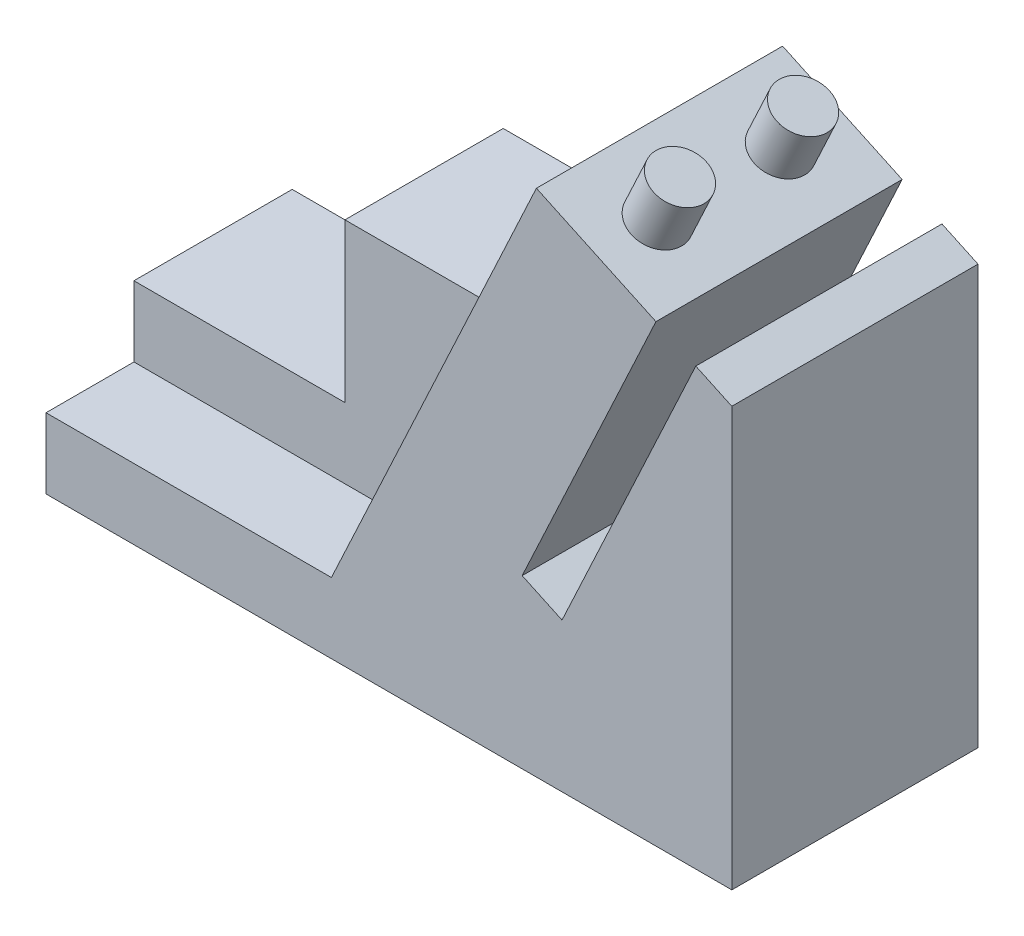
ISO-10303-21;
HEADER;
FILE_DESCRIPTION(('STEP AP214'),'2;1');
FILE_NAME('part.step','',(''),(''),'','','');
FILE_SCHEMA(('AUTOMOTIVE_DESIGN { 1 0 10303 214 1 1 1 1 }'));
ENDSEC;
DATA;
#1=APPLICATION_CONTEXT('core data for automotive mechanical design processes');
#2=APPLICATION_PROTOCOL_DEFINITION('international standard','automotive_design',2000,#1);
#3=PRODUCT_CONTEXT('',#1,'mechanical');
#4=PRODUCT('Part','Part','',(#3));
#5=PRODUCT_RELATED_PRODUCT_CATEGORY('part','',(#4));
#6=PRODUCT_DEFINITION_FORMATION('','',#4);
#7=PRODUCT_DEFINITION_CONTEXT('part definition',#1,'design');
#8=PRODUCT_DEFINITION('design','',#6,#7);
#9=PRODUCT_DEFINITION_SHAPE('','',#8);
#10=(LENGTH_UNIT() NAMED_UNIT(*) SI_UNIT(.MILLI.,.METRE.));
#11=(NAMED_UNIT(*) PLANE_ANGLE_UNIT() SI_UNIT($,.RADIAN.));
#12=(NAMED_UNIT(*) SI_UNIT($,.STERADIAN.) SOLID_ANGLE_UNIT());
#13=UNCERTAINTY_MEASURE_WITH_UNIT(LENGTH_MEASURE(1.E-05),#10,'distance_accuracy_value','');
#14=(GEOMETRIC_REPRESENTATION_CONTEXT(3) GLOBAL_UNCERTAINTY_ASSIGNED_CONTEXT((#13)) GLOBAL_UNIT_ASSIGNED_CONTEXT((#10,
#11,#12)) REPRESENTATION_CONTEXT('',''));
#15=CARTESIAN_POINT('',(0.,0.,0.));
#16=DIRECTION('',(0.,0.,1.));
#17=DIRECTION('',(1.,0.,0.));
#18=AXIS2_PLACEMENT_3D('',#15,#16,#17);
#19=CARTESIAN_POINT('',(78.,0.,28.));
#20=DIRECTION('',(0.,1.,0.));
#21=DIRECTION('',(0.,0.,1.));
#22=AXIS2_PLACEMENT_3D('',#19,#20,#21);
#23=PLANE('',#22);
#24=DIRECTION('',(1.,0.,0.));
#25=VECTOR('',#24,1.);
#26=CARTESIAN_POINT('',(78.,0.,0.));
#27=LINE('',#26,#25);
#28=CARTESIAN_POINT('',(0.,0.,0.));
#29=VERTEX_POINT('',#28);
#30=CARTESIAN_POINT('',(78.,0.,0.));
#31=VERTEX_POINT('',#30);
#32=EDGE_CURVE('E182',#29,#31,#27,.T.);
#33=ORIENTED_EDGE('',*,*,#32,.T.);
#34=DIRECTION('',(0.,0.,-1.));
#35=VECTOR('',#34,1.);
#36=CARTESIAN_POINT('',(78.,0.,28.));
#37=LINE('',#36,#35);
#38=CARTESIAN_POINT('',(78.,0.,28.));
#39=VERTEX_POINT('',#38);
#40=EDGE_CURVE('E249',#39,#31,#37,.T.);
#41=ORIENTED_EDGE('',*,*,#40,.F.);
#42=DIRECTION('',(1.,0.,0.));
#43=VECTOR('',#42,1.);
#44=CARTESIAN_POINT('',(78.,0.,28.));
#45=LINE('',#44,#43);
#46=CARTESIAN_POINT('',(0.,0.,28.));
#47=VERTEX_POINT('',#46);
#48=EDGE_CURVE('E183',#47,#39,#45,.T.);
#49=ORIENTED_EDGE('',*,*,#48,.F.);
#50=DIRECTION('',(0.,0.,-1.));
#51=VECTOR('',#50,1.);
#52=CARTESIAN_POINT('',(0.,0.,28.));
#53=LINE('',#52,#51);
#54=EDGE_CURVE('E207',#47,#29,#53,.T.);
#55=ORIENTED_EDGE('',*,*,#54,.T.);
#56=EDGE_LOOP('',(#33,#41,#49,#55));
#57=FACE_BOUND('',#56,.T.);
#58=ADVANCED_FACE('F39',(#57),#23,.F.);
#59=CARTESIAN_POINT('',(78.,47.6371964383334,28.));
#60=DIRECTION('',(-1.,0.,0.));
#61=DIRECTION('',(0.,0.,1.));
#62=AXIS2_PLACEMENT_3D('',#59,#60,#61);
#63=PLANE('',#62);
#64=DIRECTION('',(0.,1.,0.));
#65=VECTOR('',#64,1.);
#66=CARTESIAN_POINT('',(78.,47.6371964383334,0.));
#67=LINE('',#66,#65);
#68=CARTESIAN_POINT('',(78.,47.6371964383334,0.));
#69=VERTEX_POINT('',#68);
#70=EDGE_CURVE('E209',#31,#69,#67,.T.);
#71=ORIENTED_EDGE('',*,*,#70,.T.);
#72=DIRECTION('',(0.,0.,-1.));
#73=VECTOR('',#72,1.);
#74=CARTESIAN_POINT('',(78.,47.6371964383334,28.));
#75=LINE('',#74,#73);
#76=CARTESIAN_POINT('',(78.,47.6371964383334,28.));
#77=VERTEX_POINT('',#76);
#78=EDGE_CURVE('E250',#77,#69,#75,.T.);
#79=ORIENTED_EDGE('',*,*,#78,.F.);
#80=DIRECTION('',(0.,1.,0.));
#81=VECTOR('',#80,1.);
#82=CARTESIAN_POINT('',(78.,47.6371964383334,28.));
#83=LINE('',#82,#81);
#84=EDGE_CURVE('E190',#39,#77,#83,.T.);
#85=ORIENTED_EDGE('',*,*,#84,.F.);
#86=ORIENTED_EDGE('',*,*,#40,.T.);
#87=EDGE_LOOP('',(#71,#79,#85,#86));
#88=FACE_BOUND('',#87,.T.);
#89=ADVANCED_FACE('F309',(#88),#63,.F.);
#90=CARTESIAN_POINT('',(73.9030517868581,49.5476347651859,28.));
#91=DIRECTION('',(-0.422618261740702,-0.906307787036649,0.));
#92=DIRECTION('',(0.906307787036649,-0.422618261740702,0.));
#93=AXIS2_PLACEMENT_3D('',#90,#91,#92);
#94=PLANE('',#93);
#95=DIRECTION('',(-0.906307787036649,0.422618261740702,0.));
#96=VECTOR('',#95,1.);
#97=CARTESIAN_POINT('',(73.9030517868581,49.5476347651859,0.));
#98=LINE('',#97,#96);
#99=CARTESIAN_POINT('',(73.9030517868581,49.5476347651859,0.));
#100=VERTEX_POINT('',#99);
#101=EDGE_CURVE('E212',#69,#100,#98,.T.);
#102=ORIENTED_EDGE('',*,*,#101,.T.);
#103=DIRECTION('',(0.,0.,-1.));
#104=VECTOR('',#103,1.);
#105=CARTESIAN_POINT('',(73.9030517868581,49.5476347651859,28.));
#106=LINE('',#105,#104);
#107=CARTESIAN_POINT('',(73.9030517868581,49.5476347651859,28.));
#108=VERTEX_POINT('',#107);
#109=EDGE_CURVE('E242',#108,#100,#106,.T.);
#110=ORIENTED_EDGE('',*,*,#109,.F.);
#111=DIRECTION('',(-0.906307787036649,0.422618261740702,0.));
#112=VECTOR('',#111,1.);
#113=CARTESIAN_POINT('',(73.9030517868581,49.5476347651859,28.));
#114=LINE('',#113,#112);
#115=EDGE_CURVE('E188',#77,#108,#114,.T.);
#116=ORIENTED_EDGE('',*,*,#115,.F.);
#117=ORIENTED_EDGE('',*,*,#78,.T.);
#118=EDGE_LOOP('',(#102,#110,#116,#117));
#119=FACE_BOUND('',#118,.T.);
#120=ADVANCED_FACE('F304',(#119),#94,.F.);
#121=CARTESIAN_POINT('',(58.6887943641928,16.9205544318666,28.));
#122=DIRECTION('',(0.906307787036648,-0.422618261740703,0.));
#123=DIRECTION('',(0.422618261740703,0.906307787036648,0.));
#124=AXIS2_PLACEMENT_3D('',#121,#122,#123);
#125=PLANE('',#124);
#126=DIRECTION('',(-0.422618261740703,-0.906307787036648,0.));
#127=VECTOR('',#126,1.);
#128=CARTESIAN_POINT('',(58.6887943641928,16.9205544318666,0.));
#129=LINE('',#128,#127);
#130=CARTESIAN_POINT('',(58.6887943641928,16.9205544318666,0.));
#131=VERTEX_POINT('',#130);
#132=EDGE_CURVE('E214',#100,#131,#129,.T.);
#133=ORIENTED_EDGE('',*,*,#132,.T.);
#134=DIRECTION('',(0.,0.,-1.));
#135=VECTOR('',#134,1.);
#136=CARTESIAN_POINT('',(58.6887943641928,16.9205544318666,28.));
#137=LINE('',#136,#135);
#138=CARTESIAN_POINT('',(58.6887943641928,16.9205544318666,28.));
#139=VERTEX_POINT('',#138);
#140=EDGE_CURVE('E241',#139,#131,#137,.T.);
#141=ORIENTED_EDGE('',*,*,#140,.F.);
#142=DIRECTION('',(-0.422618261740703,-0.906307787036648,0.));
#143=VECTOR('',#142,1.);
#144=CARTESIAN_POINT('',(58.6887943641928,16.9205544318666,28.));
#145=LINE('',#144,#143);
#146=EDGE_CURVE('E195',#108,#139,#145,.T.);
#147=ORIENTED_EDGE('',*,*,#146,.F.);
#148=ORIENTED_EDGE('',*,*,#109,.T.);
#149=EDGE_LOOP('',(#133,#141,#147,#148));
#150=FACE_BOUND('',#149,.T.);
#151=ADVANCED_FACE('F301',(#150),#125,.F.);
#152=CARTESIAN_POINT('',(54.1572554290096,19.0336457405701,28.));
#153=DIRECTION('',(-0.422618261740703,-0.906307787036648,0.));
#154=DIRECTION('',(0.906307787036648,-0.422618261740703,0.));
#155=AXIS2_PLACEMENT_3D('',#152,#153,#154);
#156=PLANE('',#155);
#157=DIRECTION('',(-0.906307787036648,0.422618261740703,0.));
#158=VECTOR('',#157,1.);
#159=CARTESIAN_POINT('',(54.1572554290096,19.0336457405701,0.));
#160=LINE('',#159,#158);
#161=CARTESIAN_POINT('',(54.1572554290096,19.0336457405701,0.));
#162=VERTEX_POINT('',#161);
#163=EDGE_CURVE('E213',#131,#162,#160,.T.);
#164=ORIENTED_EDGE('',*,*,#163,.T.);
#165=DIRECTION('',(0.,0.,-1.));
#166=VECTOR('',#165,1.);
#167=CARTESIAN_POINT('',(54.1572554290096,19.0336457405701,28.));
#168=LINE('',#167,#166);
#169=CARTESIAN_POINT('',(54.1572554290096,19.0336457405701,28.));
#170=VERTEX_POINT('',#169);
#171=EDGE_CURVE('E238',#170,#162,#168,.T.);
#172=ORIENTED_EDGE('',*,*,#171,.F.);
#173=DIRECTION('',(-0.906307787036648,0.422618261740703,0.));
#174=VECTOR('',#173,1.);
#175=CARTESIAN_POINT('',(54.1572554290096,19.0336457405701,28.));
#176=LINE('',#175,#174);
#177=EDGE_CURVE('E191',#139,#170,#176,.T.);
#178=ORIENTED_EDGE('',*,*,#177,.F.);
#179=ORIENTED_EDGE('',*,*,#140,.T.);
#180=EDGE_LOOP('',(#164,#172,#178,#179));
#181=FACE_BOUND('',#180,.T.);
#182=ADVANCED_FACE('F300',(#181),#156,.F.);
#183=CARTESIAN_POINT('',(69.3715128516749,51.6607260738894,28.));
#184=DIRECTION('',(-0.906307787036648,0.422618261740704,0.));
#185=DIRECTION('',(-0.422618261740704,-0.906307787036648,0.));
#186=AXIS2_PLACEMENT_3D('',#183,#184,#185);
#187=PLANE('',#186);
#188=DIRECTION('',(0.422618261740704,0.906307787036648,0.));
#189=VECTOR('',#188,1.);
#190=CARTESIAN_POINT('',(69.3715128516749,51.6607260738894,0.));
#191=LINE('',#190,#189);
#192=CARTESIAN_POINT('',(69.3715128516749,51.6607260738894,0.));
#193=VERTEX_POINT('',#192);
#194=EDGE_CURVE('E219',#162,#193,#191,.T.);
#195=ORIENTED_EDGE('',*,*,#194,.T.);
#196=DIRECTION('',(0.,0.,-1.));
#197=VECTOR('',#196,1.);
#198=CARTESIAN_POINT('',(69.3715128516749,51.6607260738894,28.));
#199=LINE('',#198,#197);
#200=CARTESIAN_POINT('',(69.3715128516749,51.6607260738894,28.));
#201=VERTEX_POINT('',#200);
#202=EDGE_CURVE('E232',#201,#193,#199,.T.);
#203=ORIENTED_EDGE('',*,*,#202,.F.);
#204=DIRECTION('',(0.422618261740704,0.906307787036648,0.));
#205=VECTOR('',#204,1.);
#206=CARTESIAN_POINT('',(69.3715128516749,51.6607260738894,28.));
#207=LINE('',#206,#205);
#208=EDGE_CURVE('E198',#170,#201,#207,.T.);
#209=ORIENTED_EDGE('',*,*,#208,.F.);
#210=ORIENTED_EDGE('',*,*,#171,.T.);
#211=EDGE_LOOP('',(#195,#203,#209,#210));
#212=FACE_BOUND('',#211,.T.);
#213=ADVANCED_FACE('F263',(#212),#187,.F.);
#214=CARTESIAN_POINT('',(55.7768960461252,58.,28.));
#215=DIRECTION('',(-0.422618261740704,-0.906307787036648,0.));
#216=DIRECTION('',(0.906307787036648,-0.422618261740704,0.));
#217=AXIS2_PLACEMENT_3D('',#214,#215,#216);
#218=PLANE('',#217);
#219=CARTESIAN_POINT('',(62.5742044489,54.8303630369447,7.));
#220=DIRECTION('',(-0.422618261740704,-0.906307787036648,0.));
#221=DIRECTION('',(0.906307787036648,-0.422618261740704,0.));
#222=AXIS2_PLACEMENT_3D('',#219,#220,#221);
#223=CIRCLE('',#222,3.00000000000001);
#224=CARTESIAN_POINT('',(65.29312781001,53.5625082517226,7.));
#225=VERTEX_POINT('',#224);
#226=EDGE_CURVE('E11',#225,#225,#223,.F.);
#227=ORIENTED_EDGE('',*,*,#226,.F.);
#228=EDGE_LOOP('',(#227));
#229=FACE_BOUND('',#228,.T.);
#230=CARTESIAN_POINT('',(62.5742044489,54.8303630369447,21.));
#231=DIRECTION('',(-0.422618261740704,-0.906307787036648,0.));
#232=DIRECTION('',(0.906307787036648,-0.422618261740704,0.));
#233=AXIS2_PLACEMENT_3D('',#230,#231,#232);
#234=CIRCLE('',#233,3.);
#235=CARTESIAN_POINT('',(65.29312781001,53.5625082517226,21.));
#236=VERTEX_POINT('',#235);
#237=EDGE_CURVE('E46',#236,#236,#234,.F.);
#238=ORIENTED_EDGE('',*,*,#237,.F.);
#239=EDGE_LOOP('',(#238));
#240=FACE_BOUND('',#239,.T.);
#241=DIRECTION('',(-0.906307787036648,0.422618261740704,0.));
#242=VECTOR('',#241,1.);
#243=CARTESIAN_POINT('',(55.7768960461252,58.,0.));
#244=LINE('',#243,#242);
#245=CARTESIAN_POINT('',(55.7768960461252,58.,0.));
#246=VERTEX_POINT('',#245);
#247=EDGE_CURVE('E220',#193,#246,#244,.T.);
#248=ORIENTED_EDGE('',*,*,#247,.T.);
#249=DIRECTION('',(0.,0.,-1.));
#250=VECTOR('',#249,1.);
#251=CARTESIAN_POINT('',(55.7768960461252,58.,28.));
#252=LINE('',#251,#250);
#253=CARTESIAN_POINT('',(55.7768960461252,58.,28.));
#254=VERTEX_POINT('',#253);
#255=EDGE_CURVE('E235',#254,#246,#252,.T.);
#256=ORIENTED_EDGE('',*,*,#255,.F.);
#257=DIRECTION('',(-0.906307787036648,0.422618261740704,0.));
#258=VECTOR('',#257,1.);
#259=CARTESIAN_POINT('',(55.7768960461252,58.,28.));
#260=LINE('',#259,#258);
#261=EDGE_CURVE('E197',#201,#254,#260,.T.);
#262=ORIENTED_EDGE('',*,*,#261,.F.);
#263=ORIENTED_EDGE('',*,*,#202,.T.);
#264=EDGE_LOOP('',(#248,#256,#262,#263));
#265=FACE_BOUND('',#264,.T.);
#266=ADVANCED_FACE('F260',(#229,#240,#265),#218,.F.);
#267=CARTESIAN_POINT('',(32.461513138375,8.,28.));
#268=DIRECTION('',(0.906307787036648,-0.422618261740704,0.));
#269=DIRECTION('',(0.422618261740704,0.906307787036648,0.));
#270=AXIS2_PLACEMENT_3D('',#267,#268,#269);
#271=PLANE('',#270);
#272=DIRECTION('',(0.,0.,1.));
#273=VECTOR('',#272,1.);
#274=CARTESIAN_POINT('',(44.5855122504051,34.,28.));
#275=LINE('',#274,#273);
#276=CARTESIAN_POINT('',(44.5855122504051,34.,0.));
#277=VERTEX_POINT('',#276);
#278=CARTESIAN_POINT('',(44.5855122504051,34.,18.));
#279=VERTEX_POINT('',#278);
#280=EDGE_CURVE('E163',#277,#279,#275,.T.);
#281=ORIENTED_EDGE('',*,*,#280,.T.);
#282=DIRECTION('',(0.422618261740704,0.906307787036648,0.));
#283=VECTOR('',#282,1.);
#284=CARTESIAN_POINT('',(37.5311484498391,18.8718680098944,18.));
#285=LINE('',#284,#283);
#286=CARTESIAN_POINT('',(32.461513138375,8.,18.));
#287=VERTEX_POINT('',#286);
#288=EDGE_CURVE('E62',#287,#279,#285,.T.);
#289=ORIENTED_EDGE('',*,*,#288,.F.);
#290=DIRECTION('',(0.,0.,-1.));
#291=VECTOR('',#290,1.);
#292=CARTESIAN_POINT('',(32.461513138375,8.,28.));
#293=LINE('',#292,#291);
#294=CARTESIAN_POINT('',(32.461513138375,8.,28.));
#295=VERTEX_POINT('',#294);
#296=EDGE_CURVE('E229',#295,#287,#293,.T.);
#297=ORIENTED_EDGE('',*,*,#296,.F.);
#298=DIRECTION('',(-0.422618261740704,-0.906307787036648,0.));
#299=VECTOR('',#298,1.);
#300=CARTESIAN_POINT('',(32.461513138375,8.,28.));
#301=LINE('',#300,#299);
#302=EDGE_CURVE('E196',#254,#295,#301,.T.);
#303=ORIENTED_EDGE('',*,*,#302,.F.);
#304=ORIENTED_EDGE('',*,*,#255,.T.);
#305=DIRECTION('',(-0.422618261740704,-0.906307787036648,0.));
#306=VECTOR('',#305,1.);
#307=CARTESIAN_POINT('',(32.461513138375,8.,0.));
#308=LINE('',#307,#306);
#309=EDGE_CURVE('E221',#246,#277,#308,.T.);
#310=ORIENTED_EDGE('',*,*,#309,.T.);
#311=EDGE_LOOP('',(#281,#289,#297,#303,#304,#310));
#312=FACE_BOUND('',#311,.T.);
#313=ADVANCED_FACE('F258',(#312),#271,.F.);
#314=CARTESIAN_POINT('',(0.,8.,28.));
#315=DIRECTION('',(0.,-1.,0.));
#316=DIRECTION('',(0.,0.,-1.));
#317=AXIS2_PLACEMENT_3D('',#314,#315,#316);
#318=PLANE('',#317);
#319=ORIENTED_EDGE('',*,*,#296,.T.);
#320=DIRECTION('',(1.,0.,0.));
#321=VECTOR('',#320,1.);
#322=CARTESIAN_POINT('',(78.002,8.,18.));
#323=LINE('',#322,#321);
#324=CARTESIAN_POINT('',(0.,8.,18.));
#325=VERTEX_POINT('',#324);
#326=EDGE_CURVE('E171',#325,#287,#323,.T.);
#327=ORIENTED_EDGE('',*,*,#326,.F.);
#328=DIRECTION('',(0.,0.,-1.));
#329=VECTOR('',#328,1.);
#330=CARTESIAN_POINT('',(0.,8.,28.));
#331=LINE('',#330,#329);
#332=CARTESIAN_POINT('',(0.,8.,28.));
#333=VERTEX_POINT('',#332);
#334=EDGE_CURVE('E227',#333,#325,#331,.T.);
#335=ORIENTED_EDGE('',*,*,#334,.F.);
#336=DIRECTION('',(-1.,0.,0.));
#337=VECTOR('',#336,1.);
#338=CARTESIAN_POINT('',(0.,8.,28.));
#339=LINE('',#338,#337);
#340=EDGE_CURVE('E205',#295,#333,#339,.T.);
#341=ORIENTED_EDGE('',*,*,#340,.F.);
#342=EDGE_LOOP('',(#319,#327,#335,#341));
#343=FACE_BOUND('',#342,.T.);
#344=ADVANCED_FACE('F286',(#343),#318,.F.);
#345=CARTESIAN_POINT('',(0.,0.,28.));
#346=DIRECTION('',(1.,0.,0.));
#347=DIRECTION('',(0.,0.,-1.));
#348=AXIS2_PLACEMENT_3D('',#345,#346,#347);
#349=PLANE('',#348);
#350=DIRECTION('',(0.,-1.,0.));
#351=VECTOR('',#350,1.);
#352=CARTESIAN_POINT('',(0.,0.,0.));
#353=LINE('',#352,#351);
#354=CARTESIAN_POINT('',(0.,16.,0.));
#355=VERTEX_POINT('',#354);
#356=EDGE_CURVE('E189',#355,#29,#353,.T.);
#357=ORIENTED_EDGE('',*,*,#356,.T.);
#358=ORIENTED_EDGE('',*,*,#54,.F.);
#359=DIRECTION('',(0.,-1.,0.));
#360=VECTOR('',#359,1.);
#361=CARTESIAN_POINT('',(0.,0.,28.));
#362=LINE('',#361,#360);
#363=EDGE_CURVE('E203',#333,#47,#362,.T.);
#364=ORIENTED_EDGE('',*,*,#363,.F.);
#365=ORIENTED_EDGE('',*,*,#334,.T.);
#366=DIRECTION('',(0.,1.,0.));
#367=VECTOR('',#366,1.);
#368=CARTESIAN_POINT('',(0.,0.,18.));
#369=LINE('',#368,#367);
#370=CARTESIAN_POINT('',(0.,16.,18.));
#371=VERTEX_POINT('',#370);
#372=EDGE_CURVE('E180',#325,#371,#369,.T.);
#373=ORIENTED_EDGE('',*,*,#372,.T.);
#374=DIRECTION('',(0.,0.,-1.));
#375=VECTOR('',#374,1.);
#376=CARTESIAN_POINT('',(0.,16.,18.));
#377=LINE('',#376,#375);
#378=EDGE_CURVE('E172',#371,#355,#377,.T.);
#379=ORIENTED_EDGE('',*,*,#378,.T.);
#380=EDGE_LOOP('',(#357,#358,#364,#365,#373,#379));
#381=FACE_BOUND('',#380,.T.);
#382=ADVANCED_FACE('F278',(#381),#349,.F.);
#383=CARTESIAN_POINT('',(0.,0.,28.));
#384=DIRECTION('',(0.,0.,-1.));
#385=DIRECTION('',(-1.,0.,0.));
#386=AXIS2_PLACEMENT_3D('',#383,#384,#385);
#387=PLANE('',#386);
#388=ORIENTED_EDGE('',*,*,#48,.T.);
#389=ORIENTED_EDGE('',*,*,#84,.T.);
#390=ORIENTED_EDGE('',*,*,#115,.T.);
#391=ORIENTED_EDGE('',*,*,#146,.T.);
#392=ORIENTED_EDGE('',*,*,#177,.T.);
#393=ORIENTED_EDGE('',*,*,#208,.T.);
#394=ORIENTED_EDGE('',*,*,#261,.T.);
#395=ORIENTED_EDGE('',*,*,#302,.T.);
#396=ORIENTED_EDGE('',*,*,#340,.T.);
#397=ORIENTED_EDGE('',*,*,#363,.T.);
#398=EDGE_LOOP('',(#388,#389,#390,#391,#392,#393,#394,#395,#396,#397));
#399=FACE_BOUND('',#398,.T.);
#400=ADVANCED_FACE('F287',(#399),#387,.F.);
#401=CARTESIAN_POINT('',(0.,0.,0.));
#402=DIRECTION('',(0.,0.,-1.));
#403=DIRECTION('',(-1.,0.,0.));
#404=AXIS2_PLACEMENT_3D('',#401,#402,#403);
#405=PLANE('',#404);
#406=DIRECTION('',(-1.,0.,0.));
#407=VECTOR('',#406,1.);
#408=CARTESIAN_POINT('',(50.,34.,0.));
#409=LINE('',#408,#407);
#410=CARTESIAN_POINT('',(24.,34.,0.));
#411=VERTEX_POINT('',#410);
#412=EDGE_CURVE('E150',#277,#411,#409,.T.);
#413=ORIENTED_EDGE('',*,*,#412,.F.);
#414=ORIENTED_EDGE('',*,*,#309,.F.);
#415=ORIENTED_EDGE('',*,*,#247,.F.);
#416=ORIENTED_EDGE('',*,*,#194,.F.);
#417=ORIENTED_EDGE('',*,*,#163,.F.);
#418=ORIENTED_EDGE('',*,*,#132,.F.);
#419=ORIENTED_EDGE('',*,*,#101,.F.);
#420=ORIENTED_EDGE('',*,*,#70,.F.);
#421=ORIENTED_EDGE('',*,*,#32,.F.);
#422=ORIENTED_EDGE('',*,*,#356,.F.);
#423=DIRECTION('',(-1.,0.,0.));
#424=VECTOR('',#423,1.);
#425=CARTESIAN_POINT('',(78.002,16.,0.));
#426=LINE('',#425,#424);
#427=CARTESIAN_POINT('',(24.,16.,0.));
#428=VERTEX_POINT('',#427);
#429=EDGE_CURVE('E178',#428,#355,#426,.T.);
#430=ORIENTED_EDGE('',*,*,#429,.F.);
#431=DIRECTION('',(0.,-1.,0.));
#432=VECTOR('',#431,1.);
#433=CARTESIAN_POINT('',(24.,16.,0.));
#434=LINE('',#433,#432);
#435=EDGE_CURVE('E155',#411,#428,#434,.T.);
#436=ORIENTED_EDGE('',*,*,#435,.F.);
#437=EDGE_LOOP('',(#413,#414,#415,#416,#417,#418,#419,#420,#421,#422,#430,#436));
#438=FACE_BOUND('',#437,.T.);
#439=ADVANCED_FACE('F275',(#438),#405,.T.);
#440=CARTESIAN_POINT('',(78.002,16.,18.));
#441=DIRECTION('',(0.,1.,0.));
#442=DIRECTION('',(0.,0.,1.));
#443=AXIS2_PLACEMENT_3D('',#440,#441,#442);
#444=PLANE('',#443);
#445=DIRECTION('',(0.,0.,1.));
#446=VECTOR('',#445,1.);
#447=CARTESIAN_POINT('',(24.,16.,18.));
#448=LINE('',#447,#446);
#449=CARTESIAN_POINT('',(24.,16.,18.));
#450=VERTEX_POINT('',#449);
#451=EDGE_CURVE('E52',#428,#450,#448,.T.);
#452=ORIENTED_EDGE('',*,*,#451,.F.);
#453=ORIENTED_EDGE('',*,*,#429,.T.);
#454=ORIENTED_EDGE('',*,*,#378,.F.);
#455=DIRECTION('',(-1.,0.,0.));
#456=VECTOR('',#455,1.);
#457=CARTESIAN_POINT('',(78.002,16.,18.));
#458=LINE('',#457,#456);
#459=EDGE_CURVE('E173',#450,#371,#458,.T.);
#460=ORIENTED_EDGE('',*,*,#459,.F.);
#461=EDGE_LOOP('',(#452,#453,#454,#460));
#462=FACE_BOUND('',#461,.T.);
#463=ADVANCED_FACE('F277',(#462),#444,.T.);
#464=CARTESIAN_POINT('',(78.002,0.,18.));
#465=DIRECTION('',(0.,0.,1.));
#466=DIRECTION('',(1.,0.,0.));
#467=AXIS2_PLACEMENT_3D('',#464,#465,#466);
#468=PLANE('',#467);
#469=ORIENTED_EDGE('',*,*,#326,.T.);
#470=ORIENTED_EDGE('',*,*,#288,.T.);
#471=DIRECTION('',(-1.,0.,0.));
#472=VECTOR('',#471,1.);
#473=CARTESIAN_POINT('',(50.,34.,18.));
#474=LINE('',#473,#472);
#475=CARTESIAN_POINT('',(24.,34.,18.));
#476=VERTEX_POINT('',#475);
#477=EDGE_CURVE('E139',#279,#476,#474,.T.);
#478=ORIENTED_EDGE('',*,*,#477,.T.);
#479=DIRECTION('',(0.,1.,0.));
#480=VECTOR('',#479,1.);
#481=CARTESIAN_POINT('',(24.,16.,18.));
#482=LINE('',#481,#480);
#483=EDGE_CURVE('E144',#450,#476,#482,.T.);
#484=ORIENTED_EDGE('',*,*,#483,.F.);
#485=ORIENTED_EDGE('',*,*,#459,.T.);
#486=ORIENTED_EDGE('',*,*,#372,.F.);
#487=EDGE_LOOP('',(#469,#470,#478,#484,#485,#486));
#488=FACE_BOUND('',#487,.T.);
#489=ADVANCED_FACE('F141',(#488),#468,.T.);
#490=CARTESIAN_POINT('',(65.1099140193443,60.2682097591646,21.));
#491=DIRECTION('',(-0.422618261740704,-0.906307787036648,0.));
#492=DIRECTION('',(0.906307787036648,-0.422618261740704,0.));
#493=AXIS2_PLACEMENT_3D('',#490,#491,#492);
#494=CYLINDRICAL_SURFACE('',#493,3.);
#495=CARTESIAN_POINT('',(65.1099140193443,60.2682097591646,21.));
#496=DIRECTION('',(0.422618261740704,0.906307787036648,0.));
#497=DIRECTION('',(-0.906307787036648,0.422618261740704,0.));
#498=AXIS2_PLACEMENT_3D('',#495,#496,#497);
#499=CIRCLE('',#498,3.);
#500=CARTESIAN_POINT('',(62.3909906582343,61.5360645443867,21.));
#501=VERTEX_POINT('',#500);
#502=EDGE_CURVE('E165',#501,#501,#499,.T.);
#503=ORIENTED_EDGE('',*,*,#502,.F.);
#504=EDGE_LOOP('',(#503));
#505=FACE_BOUND('',#504,.T.);
#506=ORIENTED_EDGE('',*,*,#237,.T.);
#507=EDGE_LOOP('',(#506));
#508=FACE_BOUND('',#507,.T.);
#509=ADVANCED_FACE('F253',(#505,#508),#494,.T.);
#510=CARTESIAN_POINT('',(65.1099140193443,60.2682097591646,21.));
#511=DIRECTION('',(0.422618261740704,0.906307787036648,0.));
#512=DIRECTION('',(-0.906307787036648,0.422618261740704,0.));
#513=AXIS2_PLACEMENT_3D('',#510,#511,#512);
#514=PLANE('',#513);
#515=ORIENTED_EDGE('',*,*,#502,.T.);
#516=EDGE_LOOP('',(#515));
#517=FACE_BOUND('',#516,.T.);
#518=ADVANCED_FACE('F345',(#517),#514,.T.);
#519=CARTESIAN_POINT('',(65.1099140193443,60.2682097591646,7.));
#520=DIRECTION('',(-0.422618261740704,-0.906307787036648,0.));
#521=DIRECTION('',(0.906307787036648,-0.422618261740704,0.));
#522=AXIS2_PLACEMENT_3D('',#519,#520,#521);
#523=CYLINDRICAL_SURFACE('',#522,3.00000000000001);
#524=CARTESIAN_POINT('',(65.1099140193443,60.2682097591646,7.));
#525=DIRECTION('',(0.422618261740704,0.906307787036648,0.));
#526=DIRECTION('',(-0.906307787036648,0.422618261740704,0.));
#527=AXIS2_PLACEMENT_3D('',#524,#525,#526);
#528=CIRCLE('',#527,3.00000000000001);
#529=CARTESIAN_POINT('',(62.3909906582343,61.5360645443868,7.));
#530=VERTEX_POINT('',#529);
#531=EDGE_CURVE('E164',#530,#530,#528,.T.);
#532=ORIENTED_EDGE('',*,*,#531,.F.);
#533=EDGE_LOOP('',(#532));
#534=FACE_BOUND('',#533,.T.);
#535=ORIENTED_EDGE('',*,*,#226,.T.);
#536=EDGE_LOOP('',(#535));
#537=FACE_BOUND('',#536,.T.);
#538=ADVANCED_FACE('F343',(#534,#537),#523,.T.);
#539=CARTESIAN_POINT('',(65.1099140193443,60.2682097591646,7.));
#540=DIRECTION('',(0.422618261740704,0.906307787036648,0.));
#541=DIRECTION('',(-0.906307787036648,0.422618261740704,0.));
#542=AXIS2_PLACEMENT_3D('',#539,#540,#541);
#543=PLANE('',#542);
#544=ORIENTED_EDGE('',*,*,#531,.T.);
#545=EDGE_LOOP('',(#544));
#546=FACE_BOUND('',#545,.T.);
#547=ADVANCED_FACE('F355',(#546),#543,.T.);
#548=CARTESIAN_POINT('',(50.,34.,18.));
#549=DIRECTION('',(0.,1.,0.));
#550=DIRECTION('',(0.,0.,1.));
#551=AXIS2_PLACEMENT_3D('',#548,#549,#550);
#552=PLANE('',#551);
#553=ORIENTED_EDGE('',*,*,#280,.F.);
#554=ORIENTED_EDGE('',*,*,#412,.T.);
#555=DIRECTION('',(0.,0.,-1.));
#556=VECTOR('',#555,1.);
#557=CARTESIAN_POINT('',(24.,34.,18.));
#558=LINE('',#557,#556);
#559=EDGE_CURVE('E148',#476,#411,#558,.T.);
#560=ORIENTED_EDGE('',*,*,#559,.F.);
#561=ORIENTED_EDGE('',*,*,#477,.F.);
#562=EDGE_LOOP('',(#553,#554,#560,#561));
#563=FACE_BOUND('',#562,.T.);
#564=ADVANCED_FACE('F153',(#563),#552,.T.);
#565=CARTESIAN_POINT('',(24.,0.,0.));
#566=DIRECTION('',(-1.,0.,0.));
#567=DIRECTION('',(0.,0.,1.));
#568=AXIS2_PLACEMENT_3D('',#565,#566,#567);
#569=PLANE('',#568);
#570=ORIENTED_EDGE('',*,*,#483,.T.);
#571=ORIENTED_EDGE('',*,*,#559,.T.);
#572=ORIENTED_EDGE('',*,*,#435,.T.);
#573=ORIENTED_EDGE('',*,*,#451,.T.);
#574=EDGE_LOOP('',(#570,#571,#572,#573));
#575=FACE_BOUND('',#574,.T.);
#576=ADVANCED_FACE('F156',(#575),#569,.T.);
#577=CLOSED_SHELL('',(#58,#89,#120,#151,#182,#213,#266,#313,#344,#382,#400,#439,#463,#489,#509,
#518,#538,#547,#564,#576));
#578=MANIFOLD_SOLID_BREP('B2',#577);
#579=ADVANCED_BREP_SHAPE_REPRESENTATION('',(#18,#578),#14);
#580=SHAPE_DEFINITION_REPRESENTATION(#9,#579);
ENDSEC;
END-ISO-10303-21;
